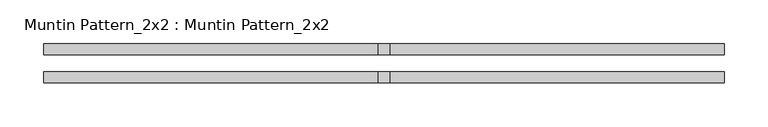
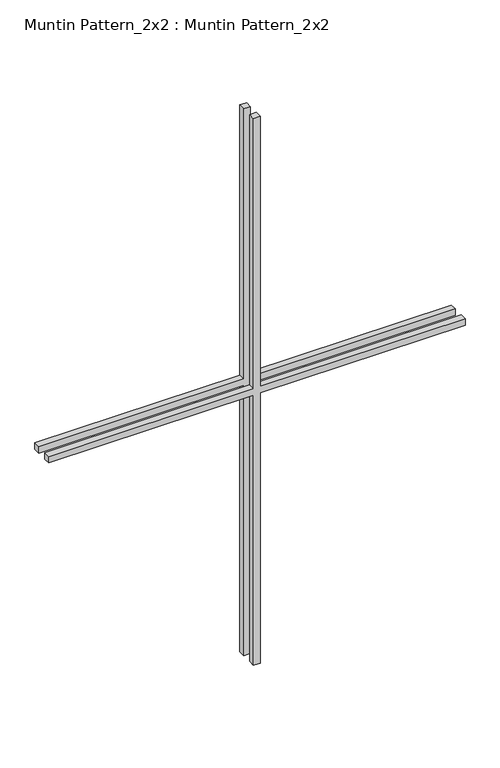
"""IFC4 building model written with IfcOpenShell, lengths in millimetres: proxy geometry, Muntin Pattern_2x2 : Muntin Pattern_2x2."""

from ifc_helpers import new_model, si_unit, frame, origin, place, context, project, spatial, polyline, outline, extrude, source, transform, mapped, element, save


def muntin_pattern_2x2_muntin_pattern_2x2_dc2504c2(model_context):
    return source(origin(), model_context, "Body", "SweptSolid", [
        extrude(outline(polyline([(546.1, -6.35), (546.1, -388.9375), (533.4, -388.9375), (533.4, -6.35), (0.0, -6.35), (0.0, 6.35), (533.4, 6.35), (533.4, 388.9375), (546.1, 388.9375), (546.1, 6.35), (1079.5, 6.35), (1079.5, -6.35), (546.1, -6.35)])), frame((0.0, 9.525, 0.0), z_axis=(0.0, 1.0, 0.0), x_axis=(0.0, 0.0, 1.0)), (0.0, 0.0, 1.0), 12.7),
        extrude(outline(polyline([(546.1, -6.35), (546.1, -388.9375), (533.4, -388.9375), (533.4, -6.35), (0.0, -6.35), (0.0, 6.35), (533.4, 6.35), (533.4, 388.9375), (546.1, 388.9375), (546.1, 6.35), (1079.5, 6.35), (1079.5, -6.35), (546.1, -6.35)])), frame((0.0, -22.225, 0.0), z_axis=(0.0, 1.0, 0.0), x_axis=(0.0, 0.0, 1.0)), (0.0, 0.0, 1.0), 12.7),
    ])


if __name__ == "__main__":
    model = new_model("IFC4")
    model_context = context("Model", 3, world=origin())
    ifc_project = project(units=[si_unit("LENGTHUNIT", "METRE", prefix="MILLI")], contexts=[model_context])
    site = spatial("IfcSite", under=ifc_project)
    building = spatial("IfcBuilding", under=site)
    placement = place(None, origin())
    muntin_pattern_2x2_muntin_pattern_2x2_shape = muntin_pattern_2x2_muntin_pattern_2x2_dc2504c2(model_context)
    element("IfcBuildingElementProxy", 1, Name="Muntin Pattern_2x2 : Muntin Pattern_2x2", ObjectType="Muntin Pattern_2x2 : Muntin Pattern_2x2", at=placement, inside=building, context=model_context, shape_type="MappedRepresentation", body=[
        mapped(muntin_pattern_2x2_muntin_pattern_2x2_shape, transform((0.0, 0.0, 0.0), x_axis=(1.0, 0.0, 0.0), y_axis=(0.0, 1.0, 0.0), z_axis=(0.0, 0.0, 1.0))),
    ])
    save(model, "model.ifc")

# Revit data of these elements
# Type "Muntin Pattern_2x2 : Muntin Pattern_2x2"
#   Width [instance default] = 4' - 0"
#   Thickness = 0' - 0 1/2"
#   Height [instance default] = 4' - 0"
#   Distance = 0' - 0 3/4"
#   Interior Material [instance default] = none
#   Exterior Material [instance default] = none
#   Default Elevation = 0
# Element 1 (IfcBuildingElementProxy, "Muntin Pattern_2x2 : Muntin Pattern_2x2")
#   Width = 2' - 6 5/8"
#   Height = 3' - 6 1/2"
#   Interior Material = Wood - Stained
#   Exterior Material = Clad - White
#   Materials on its faces: "Clad - White", "Wood - Stained"
# Materials
#   "Clad - White": class "Wood", colour RGB 242 242 238, transparency 0, Cost = 0
#   "Wood - Stained": class "Wood", colour RGB 224 178 126, transparency 0, Cost = 0
